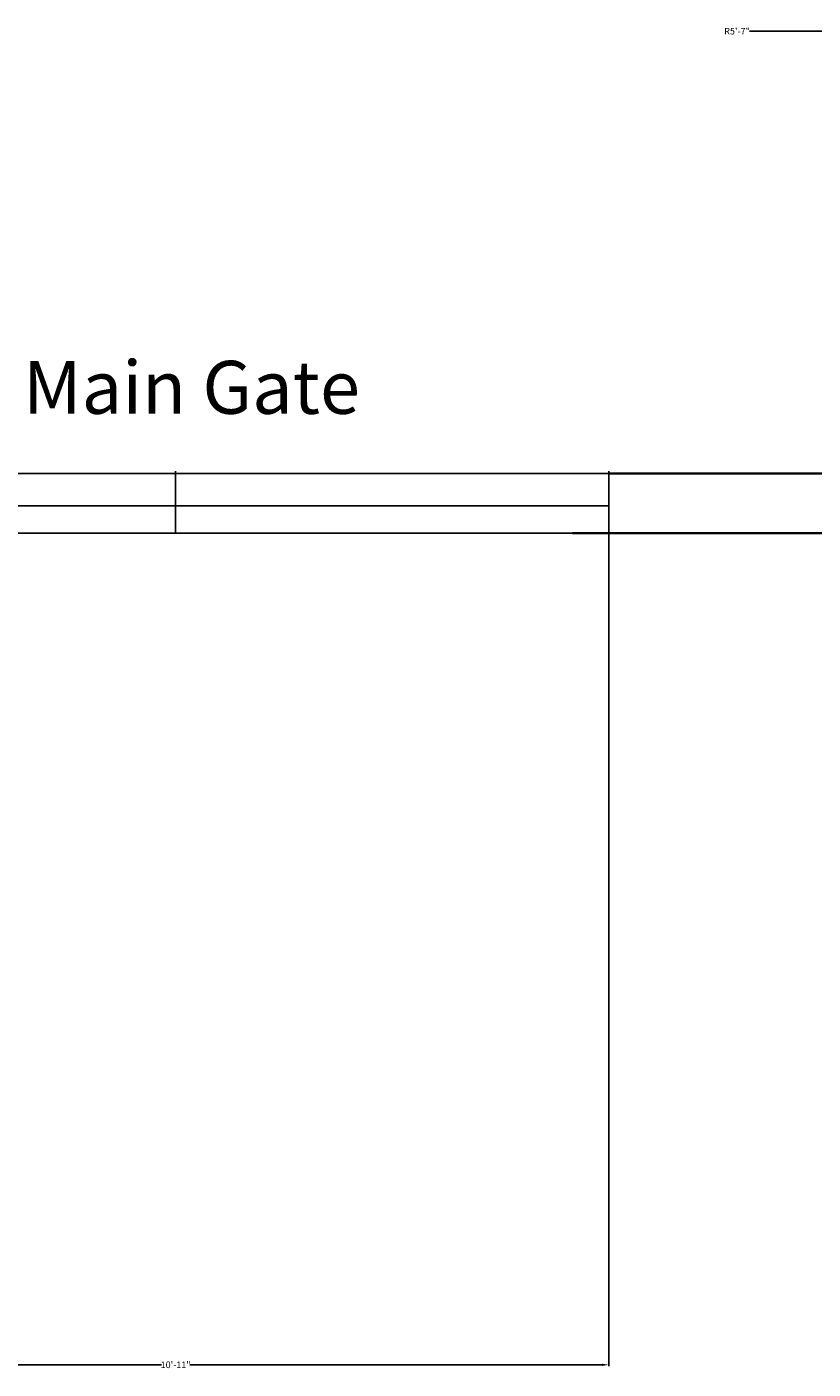
# Model space of a CAD drawing. Units: inches. Extents: x 371 to 1095, y -45 to 1219.
# Tile 2 of 18: x 740 to 859, y -44 to 159. Entities that reach past the tile are written whole.
import ezdxf

# ---------------------------------------------------------------- set-up
doc = ezdxf.new("R2010")
doc.units = ezdxf.units.IN
doc.header["$MEASUREMENT"] = 0
for name, color, linetype, lineweight in [('A-ANNO-DIMS', 2, 'Continuous', 18), ('A-ANNO-TEXT', 7, 'Continuous', 18), ('C-SITE-GATE', 3, 'Continuous', 25), ('C-SITE-WALL', 40, 'Continuous', 35)]:
    doc.layers.add(name, color=color, linetype=linetype, lineweight=lineweight)
doc.styles.get("Standard").update_dxf_attribs({"font": 'arial.ttf'})
doc.dimstyles.get("Standard").update_dxf_attribs({"dimtxt": 1, "dimasz": 1, "dimexe": 0.18, "dimexo": 0.0625, "dimgap": 0.09, "dimtad": 0, "dimtih": 1, "dimtoh": 1, "dimdec": 0, "dimzin": 0, "dimdsep": 46, "dimlunit": 3, "dimtxsty": 'Standard', "dimcen": 0.09, "dimadec": 0, "dimazin": 0, "dimtfac": 1, "dimtdec": 0, "dimtofl": 0, "dimtmove": 0, "dimatfit": 3, "dimfxl": 1, "dimtolj": 1, "dimtzin": 0, "dimarcsym": 0})

# ---------------------------------------------------------------- blocks, each defined once
blk = doc.blocks.new('*U18')
for p, q in [((-28, 0), (-28, -4)), ((0, 0), (0, -4))]:
    blk.add_line(p, q)
blk.add_lwpolyline([(0, 0), (-28, 0), (-28, -1.75), (0, -1.75)], close=True)
blk = doc.blocks.new('*D52')
at = {"layer": 'A-ANNO-DIMS', "color": 0, "lineweight": -2, "transparency": 16777216}
for p, q in [((697.33, 81.96), (697.33, -43.83)), ((828.28, 81.96), (828.28, -43.83)), ((698.33, -43.65), (760.66, -43.65)), ((827.28, -43.65), (764.96, -43.65))]:
    blk.add_line(p, q, dxfattribs=at)
at = {"layer": 'A-ANNO-DIMS', "color": 0, "transparency": 16777216}
for points in [[(698.33, -43.48), (698.33, -43.82), (697.33, -43.65)], [(827.28, -43.48), (827.28, -43.82), (828.28, -43.65)]]:
    blk.add_solid(points, dxfattribs=at)
at = {"layer": 'Defpoints', "color": 0, "transparency": 16777216}
for p in [(697.33, 82.03), (828.28, 82.03), (828.28, -43.65)]:
    blk.add_point(p, dxfattribs=at)
at = {"layer": 'A-ANNO-DIMS', "color": 0, "transparency": 16777216, "insert": (762.81, -43.65), "char_height": 1, "attachment_point": 5}
blk.add_mtext('\\A1;10\'-11"', dxfattribs=at)
blk = doc.blocks.new('*D66')
at = {"layer": 'A-ANNO-DIMS', "color": 0, "lineweight": -2, "transparency": 16777216}
for p, q in [((849.55, 157.87), (888.76, 157.87)), ((956.69, 157.87), (956.87, 157.87)), ((956.78, 157.78), (956.78, 157.96))]:
    blk.add_line(p, q, dxfattribs=at)
at = {"layer": 'A-ANNO-DIMS', "color": 0, "transparency": 16777216}
blk.add_solid([(888.76, 158.03), (888.76, 157.7), (889.76, 157.87)], dxfattribs=at)
at = {"layer": 'Defpoints', "color": 0, "transparency": 16777216}
for p in [(889.76, 157.87), (956.78, 157.87)]:
    blk.add_point(p, dxfattribs=at)
at = {"layer": 'A-ANNO-DIMS', "color": 0, "transparency": 16777216, "insert": (847.66, 157.87), "char_height": 1, "attachment_point": 5}
blk.add_mtext('\\A1;R5\'-7"', dxfattribs=at)

msp = doc.modelspace()

# ---------------------------------------------------------------- linework, layer by layer
at = {"layer": 'C-SITE-GATE'}
for p, q in [((697.33, 91.03), (828.28, 91.03)), ((762.81, 91.03), (762.81, 82.03))]:
    msp.add_line(p, q, dxfattribs=at)
at = {"layer": 'C-SITE-WALL'}
for p, q in [((828.28, 91.03), (1023.81, 91.03)), ((822.81, 82.03), (1032.81, 82.03))]:
    msp.add_line(p, q, dxfattribs=at)

# ---------------------------------------------------------------- block references
at = {"layer": 'C-SITE-GATE', "yscale": 2.338360003491396, "zscale": 2.338360003491396, "rotation": 180}
for p, xscale in [((697.33, 82.03), 2.338360003491396), ((828.28, 82.03), -2.338360003491396)]:
    msp.add_blockref('*U18', p, dxfattribs=dict(at, xscale=xscale))

# ---------------------------------------------------------------- texts
at = {"layer": 'A-ANNO-TEXT', "insert": (739.74, 108.05), "char_height": 8, "attachment_point": 1}
msp.add_mtext_dynamic_manual_height_columns('Main Gate', width=113.4312, gutter_width=1, heights=[0], dxfattribs=at)

# ---------------------------------------------------------------- dimensions: what is measured, and where the dimension line sits
at = {"layer": 'A-ANNO-DIMS'}
dim = msp.add_radius_dim(center=(956.78, 157.87), mpoint=(889.76, 157.87), dimstyle='Standard', override={"dimdec": 1, "dimlfac": 1, "dimrnd": 0, "dimzin": 1, "dimdsep": 46, "dimlunit": 4, "dimfrac": 2}, dxfattribs=at)
dim.commit()
dim.dimension.update_dxf_attribs({"geometry": '*D66', "text_midpoint": (849.55, 157.87), "dimtype": 164})
dim = msp.add_linear_dim(base=(828.282, -43.649), p1=(697.3338, 82.0251), p2=(828.282, 82.0251), dimstyle='Standard', override={"dimdec": 1, "dimlfac": 1, "dimrnd": 0, "dimzin": 1, "dimdsep": 46, "dimlunit": 4, "dimfrac": 2}, dxfattribs=at)
dim.commit()
dim.dimension.update_dxf_attribs({"geometry": '*D52', "text_midpoint": (762.8079, -43.649)})

doc.saveas('drawing.dxf')
